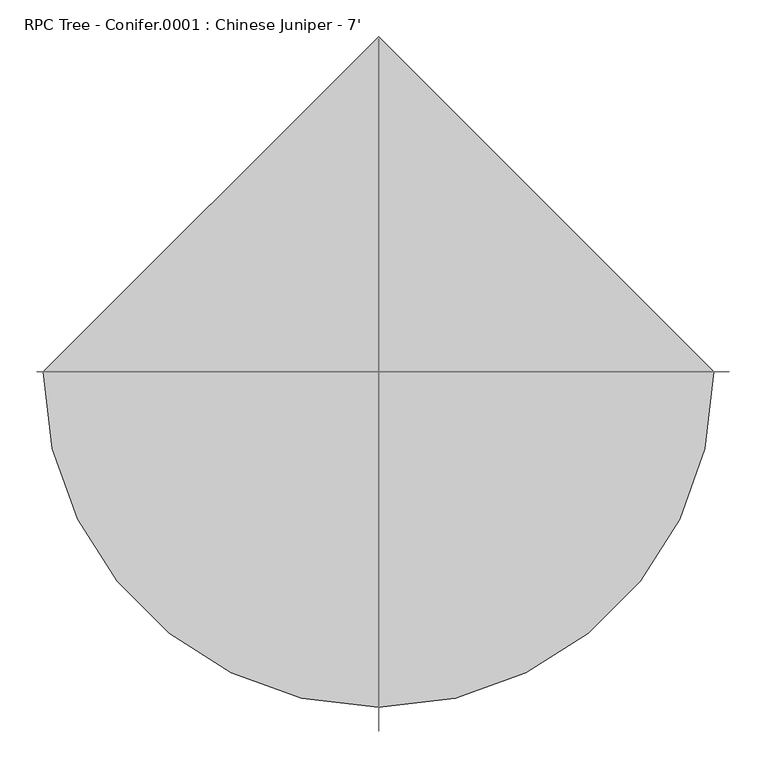
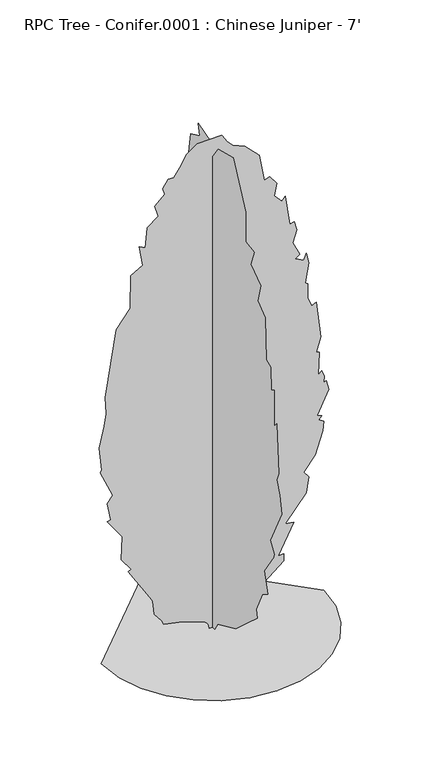
"""IFC4 building model written with IfcOpenShell, lengths in millimetres: geographic element geometry, RPC Tree - Conifer.0001 : Chinese Juniper - 7'."""

from ifc_helpers import new_model, si_unit, origin, place, context, project, spatial, triangles, source, transform, mapped, element, save


def rpc_tree_conifer_0001_chinese_juniper_7_1b9786cd(model_context):
    return source(origin(), model_context, "Body", "Tessellation", [
        triangles([(-14.517647, 6e-07, 1.3e-06), (-18.0071097, -3e-07, 17.9396969), (-27.4223632, -6e-07, 30.3914521), (-123.5685295, 1.5e-06, 65.7757953), (-201.676062, 3.9e-06, 82.3498608), (-209.1624873, 3.1e-06, 101.0656516), (-239.326362, 2.1e-06, 139.6788561), (-246.5945957, -1e-06, 198.3880905), (-257.8249785, -1.9e-06, 220.8470939), (-347.6599566, -6.4e-06, 363.0865585), (-336.0369015, -7.4e-06, 370.071561), (-375.7854927, -8.9e-06, 425.7942498), (-371.7570322, -1.5e-05, 524.6285151), (-433.7535387, -1.74e-05, 610.1379032), (-418.7802157, -1.83e-05, 613.8793173), (-433.1718882, -2.22e-05, 689.5207758), (-411.2922644, -2.49e-05, 718.6876728), (-463.6977139, -2.95e-05, 834.7279736), (-456.2123059, -3.02e-05, 842.2133451), (-467.4416714, -3.58e-05, 943.2777431), (-447.126705, -4.19e-05, 1031.4541197), (-437.4949891, -4.53e-05, 1081.7767748), (-441.2389466, -4.94e-05, 1152.8969976), (-396.3214485, -6.81e-05, 1433.6338589), (-340.174585, -7.5e-05, 1508.4981846), (-337.1392688, -8.35e-05, 1648.2265743), (-287.7691355, -8.74e-05, 1676.941246), (-302.7424948, -9.18e-05, 1763.0323574), (-277.1874594, -9.21e-05, 1748.371479), (-269.0543621, -9.76e-05, 1834.1525803), (-224.1350836, -0.0001015, 1867.8406403), (-239.107916, -0.0001038, 1916.5022049), (-197.9328675, -0.0001078, 1953.9342224), (-205.4192747, -0.000109, 1980.1369835), (-182.9602713, -0.000112, 2013.8251888), (-160.5012679, -0.000113, 2013.8251888), (-134.7328734, -0.0001161, 2047.2821583), (-108.898967, -0.0001202, 2095.8470718), (-62.5486394, -0.0001241, 2127.2339642), (37.1144179, -0.0001285, 2128.801165), (60.3458442, -0.0001273, 2092.4307106), (82.8048476, -0.000127, 2069.9720524), (132.737601, -0.0001279, 2048.8239246), (191.3566519, -0.0001268, 1987.6224277), (213.8156735, -0.0001209, 1871.5845978), (236.2746769, -0.0001223, 1879.070042), (263.6666277, -0.0001212, 1839.8828991), (254.989959, -0.0001178, 1789.2351185), (284.9366594, -0.0001171, 1755.5469131), (299.9074571, -0.0001186, 1770.5202724), (318.6248102, -0.0001119, 1643.2505699), (337.3395836, -0.0001129, 1646.9946728), (347.517378, -0.0001111, 1609.9130699), (330.7888933, -0.0001074, 1559.0291119), (359.7983145, -0.000105, 1497.2687828), (340.1843954, -0.0001034, 1485.5084541), (374.7716738, -0.0001038, 1467.3220642), (386.0010392, -0.0001059, 1493.5248253), (397.230441, -0.0001037, 1448.6072182), (382.2596251, -9.81e-05, 1366.2577389), (393.0673594, -9.81e-05, 1357.3651131), (391.5662155, -9.44e-05, 1296.562429), (408.4598064, -9.28e-05, 1257.7053532), (427.1771233, -9.41e-05, 1265.1907974), (445.8918966, -8.55e-05, 1107.9794632), (427.1771233, -8.11e-05, 1048.0886421), (438.8332068, -8.14e-05, 1044.1287821), (434.6625312, -7.54e-05, 947.0217007), (449.6358905, -7.68e-05, 958.2511024), (460.8652559, -7.57e-05, 932.0483414), (457.1212984, -7.4e-05, 905.8481964), (468.3506639, -7.47e-05, 909.5896105), (479.5800293, -7.27e-05, 868.4161062), (430.9185737, -6.48e-05, 771.0931223), (449.6358905, -6.52e-05, 763.6077507), (438.4064887, -6.38e-05, 748.6343914), (457.1212984, -6.39e-05, 737.4049896), (453.1842567, -6.13e-05, 697.0620306), (423.4331657, -5.44e-05, 602.6499518), (374.7716738, -4.87e-05, 542.7590944), (397.230441, -4.81e-05, 516.5563697), (384.9545551, -4.37e-05, 451.166393), (299.9074571, -3.36e-05, 344.3717488), (333.5981332, -3.49e-05, 340.6277913), (269.9633001, -2.47e-05, 217.1038994), (292.4220673, -2.57e-05, 217.1038994), (292.4220673, -2.39e-05, 187.1584707), (127.7223548, -8.7e-06, 52.4044321), (127.7223548, -9.8e-06, 71.1202274), (15.4277284, -7e-07, 0.0), (0.1966721, 13.7891713, 0.00013), (0.1966737, 34.4811189, 14.2963339), (0.1966762, 77.4229995, 29.9456808), (0.1966783, 178.488651, 67.3772736), (0.1966827, 230.8930831, 116.0384931), (0.1966819, 208.4340797, 119.7817057), (0.1966904, 288.5449239, 235.2565704), (0.1966918, 264.5824875, 291.9663175), (0.196695, 331.9587347, 389.2892833), (0.1966967, 324.4733268, 434.2067814), (0.1967014, 373.1322753, 494.0976388), (0.1967052, 389.4924685, 565.7309481), (0.1967041, 380.6202267, 640.0820784), (0.1967106, 440.5110841, 729.9170746), (0.1967147, 444.2524981, 819.7546143), (0.196717, 422.6319428, 893.2725832), (0.1967196, 455.4818636, 1010.6565519), (0.19672, 425.5377248, 1051.8300562), (0.1967236, 388.1056346, 1171.611771), (0.1967244, 414.3083593, 1253.9613956), (0.1967283, 384.3616407, 1373.7430378), (0.1967298, 346.932094, 1444.8632607), (0.1967315, 328.2147772, 1594.5917667), (0.19673, 305.75601, 1583.362365), (0.1967359, 305.75601, 1718.1148956), (0.1967344, 260.8385118, 1729.3441521), (0.1967329, 237.0752094, 1809.303661), (0.1967352, 223.406676, 1875.3287006), (0.1967352, 178.488651, 1920.2461624), (0.1967401, 156.0296476, 2055.0011639), (0.1967346, 92.3955867, 2084.9454117), (0.1967371, 102.0598133, 2133.1292439), (0.1967319, 11.3487565, 2104.2112415), (0.1967329, 6.3027505, 2040.0278046), (0.1967297, -38.6152347, 2103.6627285), (0.1967262, -147.1670527, 2133.606831), (0.1967183, -237.0033388, 1950.1902649), (0.1967127, -237.0033388, 1822.9231785), (0.1967097, -296.2055936, 1812.3847229), (0.1967078, -270.691199, 1744.3175114), (0.1967065, -342.8426634, 1695.0642677), (0.196704, -323.0966666, 1617.050425), (0.1966999, -375.4995727, 1575.8744499), (0.1966957, -382.9874877, 1396.2018414), (0.1966938, -413.5488853, 1383.1639744), (0.1966894, -416.6756204, 1283.9081142), (0.196689, -439.1343876, 1298.8788574), (0.1966862, -439.1343876, 1141.6675959), (0.1966823, -457.849161, 1164.1263994), (0.1966765, -472.8225203, 954.5096884), (0.1966757, -456.5690065, 918.855542), (0.1966723, -480.3104716, 864.672076), (0.1966725, -491.5398371, 789.8078957), (0.1966689, -412.9316628, 628.8526766), (0.1966658, -439.1343876, 583.9351785), (0.1966692, -436.9195155, 568.0778978), (0.1966679, -368.0141647, 467.8974212), (0.1966629, -394.2168895, 381.8038754), (0.1966636, -353.0408054, 355.6011506), (0.1966655, -311.8672648, 265.7661362), (0.1966637, -319.3526728, 232.0767318), (0.196664, -244.4894916, 164.6997216), (0.1966643, -165.8828434, 93.5794897), (0.1966675, -34.8715179, 33.6886368), (0.1966708, -16.1562041, 0.0001282), (-457.9674314, 0.0, 0.0001492), (-445.8541446, -104.9808196, 0.0001424), (-411.358285, -201.3891246, 0.0001352), (-357.2408761, -286.4621113, 0.0001277), (-286.2654482, -357.4375574, 0.0001204), (-201.1924614, -411.5549664, 0.0001134), (-104.7841473, -446.0508259, 0.0001072), (0.1966917, -458.1641127, 0.0001019), (105.1774918, -446.0508259, 9.8e-05), (201.5857877, -411.5549664, 9.58e-05), (286.6587745, -357.4375574, 9.54e-05), (357.6342387, -286.4621113, 9.65e-05), (411.7516477, -201.3888702, 9.92e-05), (446.2475072, -104.9808196, 0.0001034), (458.360794, 4.01e-05, 0.0001092), (0.1966112, 458.1641127, 0.0001565)], [[57, 58, 59], [27, 28, 29], [87, 88, 89], [49, 50, 51], [13, 14, 15], [83, 84, 85], [74, 75, 76], [63, 64, 65], [68, 69, 70], [71, 72, 73], [9, 10, 11], [85, 86, 87], [85, 87, 89], [51, 52, 53], [54, 55, 56], [90, 1, 2], [66, 67, 68], [45, 46, 47], [17, 18, 19], [68, 70, 71], [45, 47, 48], [31, 32, 33], [76, 77, 78], [89, 90, 2], [89, 2, 3], [57, 59, 60], [51, 53, 54], [25, 26, 27], [39, 40, 41], [56, 57, 60], [71, 73, 74], [34, 35, 36], [33, 34, 36], [4, 5, 6], [60, 61, 62], [80, 81, 82], [38, 39, 41], [37, 38, 41], [37, 41, 42], [29, 30, 31], [15, 16, 17], [36, 37, 42], [33, 36, 42], [31, 33, 42], [31, 42, 43], [31, 43, 44], [31, 44, 45], [29, 31, 45], [29, 45, 48], [27, 29, 48], [25, 27, 48], [25, 48, 49], [25, 49, 51], [25, 51, 54], [25, 54, 56], [25, 56, 60], [25, 60, 62], [24, 25, 62], [23, 24, 62], [22, 23, 62], [22, 62, 63], [22, 63, 65], [22, 65, 66], [22, 66, 68], [21, 22, 68], [20, 21, 68], [19, 20, 68], [17, 19, 68], [17, 68, 71], [17, 71, 74], [15, 17, 74], [13, 15, 74], [13, 74, 76], [13, 76, 78], [13, 78, 79], [13, 79, 80], [12, 13, 80], [11, 12, 80], [9, 11, 80], [9, 80, 82], [9, 82, 83], [9, 83, 85], [9, 85, 89], [9, 89, 3], [9, 3, 4], [8, 9, 4], [8, 4, 6], [7, 8, 6], [138, 139, 140], [94, 95, 96], [136, 137, 138], [121, 122, 123], [112, 113, 114], [128, 129, 130], [121, 123, 124], [125, 126, 127], [124, 125, 127], [114, 115, 116], [147, 148, 149], [130, 131, 132], [124, 127, 128], [134, 135, 136], [154, 155, 91], [154, 91, 92], [150, 151, 152], [96, 97, 98], [119, 120, 121], [119, 121, 124], [119, 124, 128], [118, 119, 128], [117, 118, 128], [116, 117, 128], [116, 128, 130], [114, 116, 130], [114, 130, 132], [112, 114, 132], [112, 132, 133], [112, 133, 134], [112, 134, 136], [111, 112, 136], [110, 111, 136], [109, 110, 136], [109, 136, 138], [109, 138, 140], [109, 140, 141], [108, 109, 141], [107, 108, 141], [106, 107, 141], [105, 106, 141], [104, 105, 141], [103, 104, 141], [103, 141, 142], [103, 142, 143], [103, 143, 144], [102, 103, 144], [101, 102, 144], [100, 101, 144], [100, 144, 145], [100, 145, 146], [100, 146, 147], [100, 147, 149], [100, 149, 150], [100, 150, 152], [100, 152, 153], [100, 153, 154], [99, 100, 154], [98, 99, 154], [96, 98, 154], [96, 154, 92], [96, 92, 93], [96, 93, 94], [170, 171, 156], [169, 170, 156], [169, 156, 157], [168, 169, 157], [168, 157, 158], [168, 158, 159], [167, 168, 159], [166, 167, 159], [166, 159, 160], [166, 160, 161], [166, 161, 162], [166, 162, 163], [166, 163, 164], [166, 164, 165]], closed=False),
    ])


if __name__ == "__main__":
    model = new_model("IFC4")
    model_context = context("Model", 3, world=origin())
    ifc_project = project(units=[si_unit("LENGTHUNIT", "METRE", prefix="MILLI")], contexts=[model_context])
    site = spatial("IfcSite", under=ifc_project)
    building = spatial("IfcBuilding", under=site)
    placement = place(None, origin())
    rpc_tree_conifer_0001_chinese_juniper_7_shape = rpc_tree_conifer_0001_chinese_juniper_7_1b9786cd(model_context)
    element("IfcGeographicElement", 1, ObjectType="RPC Tree - Conifer.0001 : Chinese Juniper - 7'", at=placement, inside=building, context=model_context, shape_type="MappedRepresentation", body=[
        mapped(rpc_tree_conifer_0001_chinese_juniper_7_shape, transform((0.0, 0.0, 0.0), x_axis=(1.0, 0.0, 0.0), y_axis=(0.0, 1.0, 0.0), z_axis=(0.0, 0.0, 1.0))),
    ])
    save(model, "model.ifc")

# Revit data of these elements
# Type "RPC Tree - Conifer.0001 : Chinese Juniper - 7'"
#   built-in parameter 1005198 = "{2, 15},{39, RPC-16-FUM3-UUQ0-UBF0-N000-ST1L-LVER-AU},{1, 0},{1, 0},{2, 13},{1, 8},{5, Color},{1, 0},{1, 0},{3, 0.8},{3, 0.8},{3, 0.8},{1, 8},{7, BBoxMin},{1, 0},{1, 0},{1, 0},{1, 0},{1, 0},{1, 8},{7, BBoxMax},{1, 0},{1, 0},{1, 0},{1, 0},{1, 0},{2, 11},{9, RPCTypeId},{1, 0},{1, 0},{39, RPC-16-FUM3-UUQ0-UBF0-N000-ST1L-LVER-AU},{1, 6},{14, RPCPlantHeight},{1, 0},{1, 0},{1, 7},{2, 11},{7, keyword},{1, 0},{1, 0},{34, :RPCs:Trees [General]:Geometry:RPC},{2, 11},{8, category},{1, 0},{1, 0},{15, Trees [General]},{2, 11},{12, LocalizedUID},{1, 0},{1, 0},{15, Chinese Juniper},{2, 14},{6, Height},{1, 0},{1, 0},{1, 7},{1, 2},{16, Cast Reflections},{1, 0},{1, 0},{1, 0},{1, 2},{12, Cast Shadows},{1, 0},{1, 0},{1, 1},{1, 2},{9, Lock View},{1, 0},{1, 0},{1, 0},{1, 4},{5, ViewC},{1, 0},{1, 0},{1, 0},{21, assetlibrary_base.fbx},{1, 5},"
#   built-in parameter 1005195 = "RPC-16-FUM3-UUQ0-UBF0-N000-ST1L-LVER-AU"
#   Type Comments = "Chinese Juniper"
#   Assembly Code = "G2050500"
#   Height = 7' - 0"
#   Description = (empty or 0)
#   Default Elevation = 0
